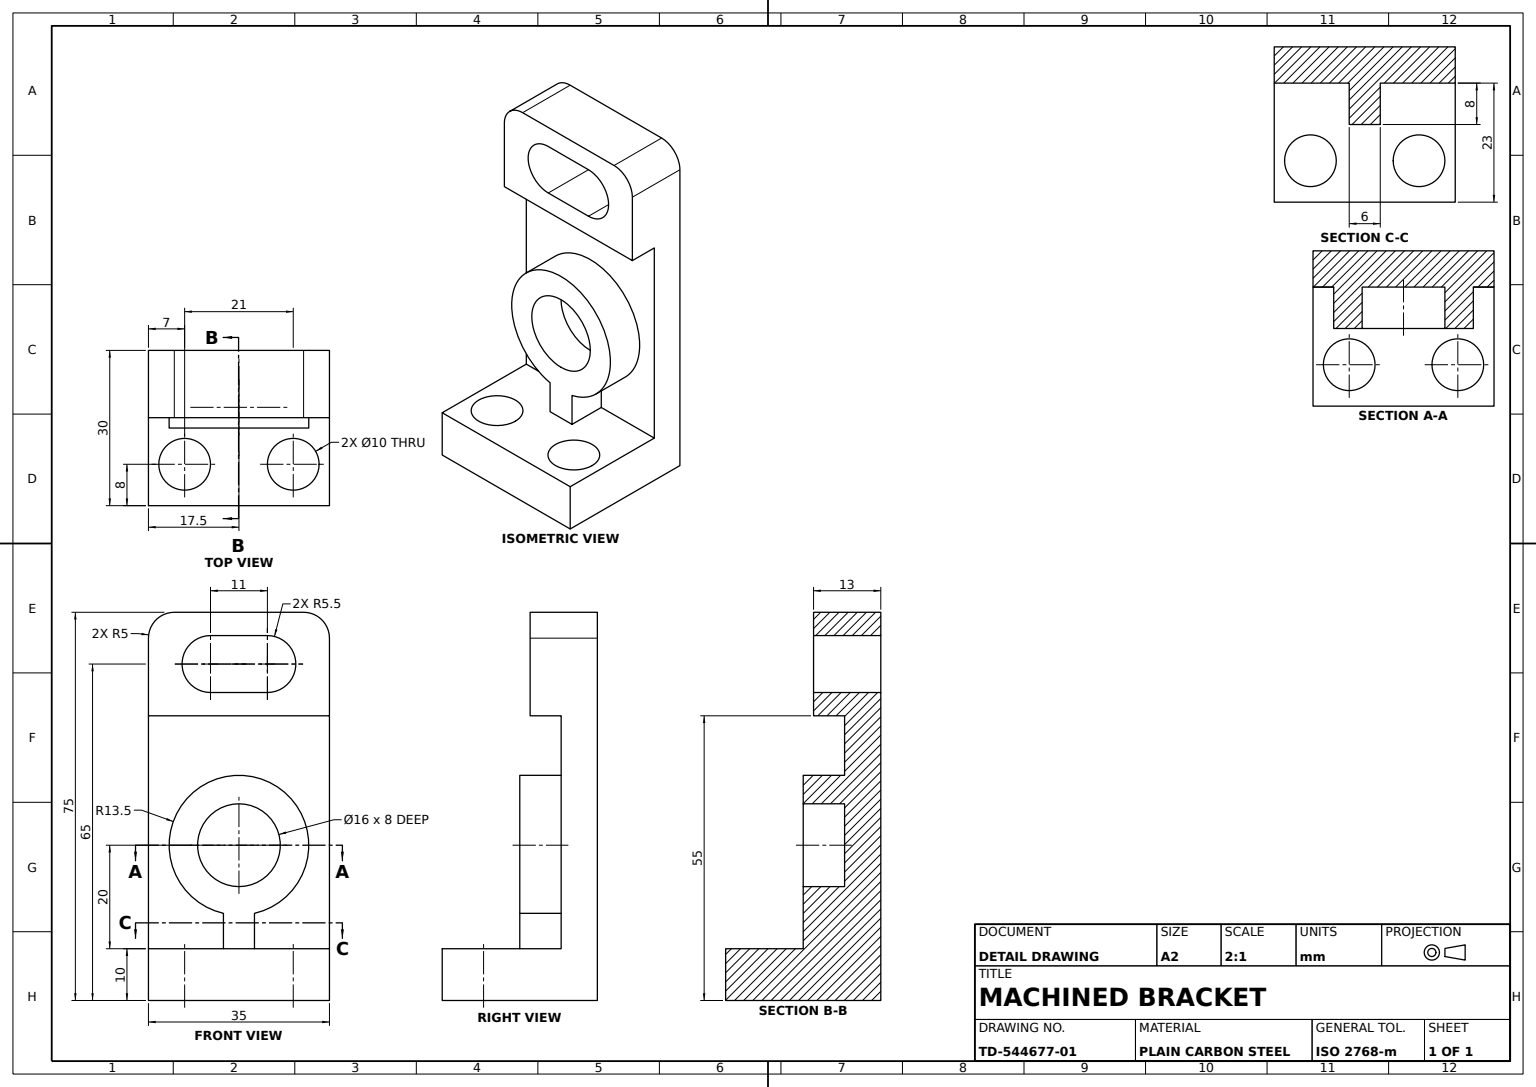
SolidWorks part; units mm, degrees
material "Plain Carbon Steel"
ref_plane "Front Plane" through (0, 0, 0) normal (0, 0, 1) x (1, 0, 0)
ref_plane "Top Plane" through (0, 0, 0) normal (0, 1, 0) x (1, 0, 0)
ref_plane "Right Plane" through (0, 0, 0) normal (1, 0, 0) x (0, 0, -1)
sketch "Bracket Profile Sketch" plane through (0, 0, 0) normal (0, 0, 1) x (1, 0, 0)
  line L0 (0, 0) -> (0, 75)
  line L1 (0, 75) -> (13, 75)
  line L2 (13, 75) -> (13, 55)
  line L3 (13, 55) -> (7, 55)
  line L4 (7, 55) -> (7, 10)
  line L5 (7, 10) -> (30, 10)
  line L6 (30, 10) -> (30, 0)
  line L7 (30, 0) -> (0, 0)
  dimension "D1" = 30
  dimension "D2" = 23
  dimension "D3" = 10
  dimension "D4" = 13
  dimension "D5" = 75
  dimension "D6" = 55
extrude "Bracket Body" add sketch "Bracket Profile Sketch" against normal blind 35
sketch "Base Holes Sketch" plane through (0, 10, 0) normal (0, 1, 0) x (1, 0, 0)
  line L0 (0, 17.5) -> (32.2005, 17.5) construction
  line L1 (0, 35) -> (0, 0) construction
  line L3 (30, 35) -> (30, 0) construction
  circle A0 centre (22, 28) radius 5
  circle A1 centre (22, 7) radius 5
  dimension "D1" = 10
  dimension "D2" = 21
  dimension "D3" = 8
extrude "Base Holes Cut" cut sketch "Base Holes Sketch" against normal up to next
sketch "Ring Boss Sketch" plane through (7, 0, 0) normal (1, 0, 0) x (0, 0, -1)
  line L0 (35, 0) -> (0, 0) construction
  line L1 (14.5, 16.8376) -> (14.5, 10)
  line L2 (35, 10) -> (0, 10) construction
  line L3 (20.5, 16.8376) -> (20.5, 10)
  line L4 (17.5, 61.6732) -> (17.5, -4.3687) construction
  line L5 (14.5, 10) -> (20.5, 10)
  circle A0 centre (17.5, 30) radius 8
  arc A1 (20.5, 16.8376) -> (14.5, 16.8376) centre (17.5, 30) ccw
  point P2 (17.5, 10)
  point P5 (17.5, 0)
  dimension "D1" = 27
  dimension "D2" = 16
  dimension "D3" = 6
  dimension "D4" = 20
extrude "Ring Boss" add sketch "Ring Boss Sketch" along normal blind 8
fillet "Top Edge Fillet R5" radius 5 2 edges at (6.5, 75, -35) (6.5, 75, 0)
sketch "Top Slot Sketch" plane through (13, 0, 0) normal (1, 0, 0) x (0, 0, -1)
  line L0 (12, 70.5) -> (23, 70.5)
  line L1 (23, 59.5) -> (12, 59.5)
  line L2 (17.5, 75) -> (17.5, 46.1837) construction
  line L3 (30, 75) -> (5, 75) construction
  arc A0 (12, 70.5) -> (12, 59.5) centre (12, 65) ccw
  arc A1 (23, 59.5) -> (23, 70.5) centre (23, 65) ccw
  dimension "D1" = 11
  dimension "D2" = 11
  dimension "D3" = 65
extrude "Top Slot Cut" cut sketch "Top Slot Sketch" against normal up to next
